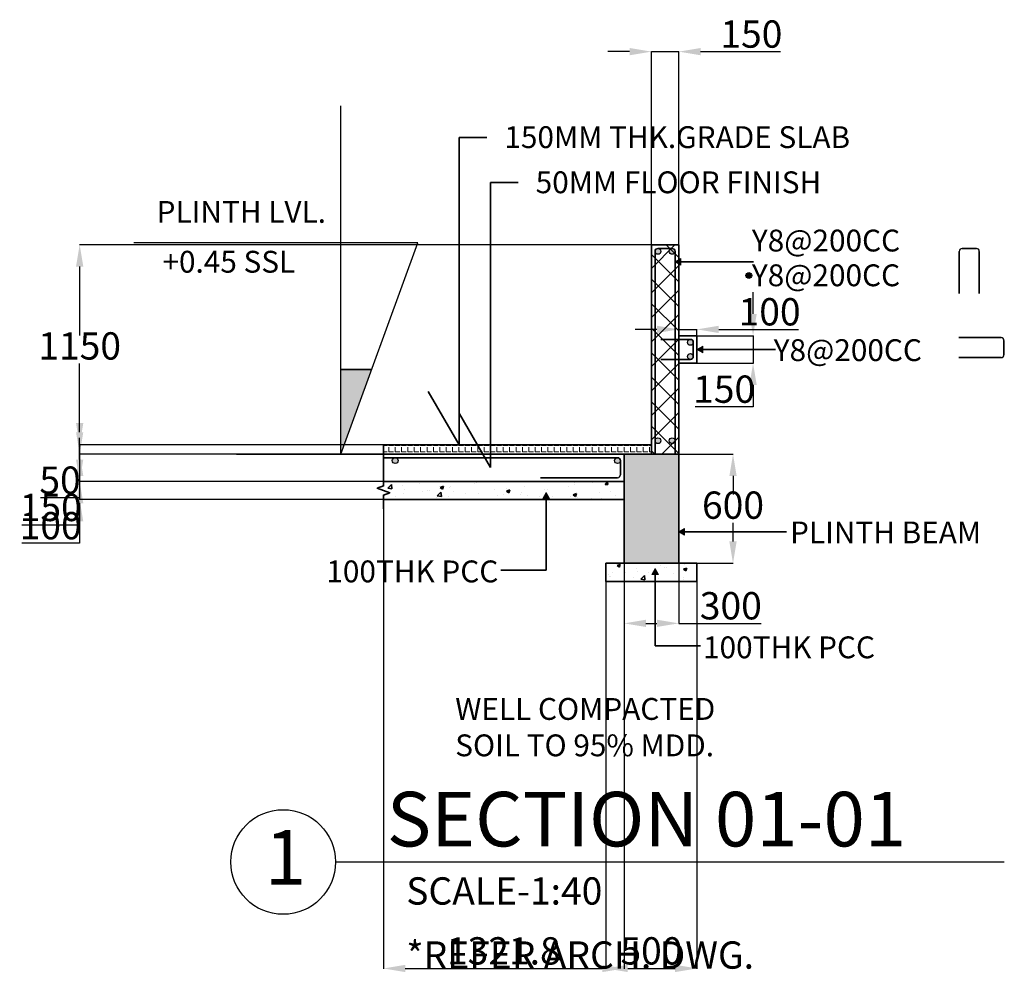
# Model space of a CAD drawing. Units: millimetres. Extents: x -174 to 32373, y 27344 to 53129.
# Tile 1 of 7: x -174 to 5234, y 30305 to 35540. Entities that reach past the tile are written whole.
import ezdxf

# ---------------------------------------------------------------- set-up
doc = ezdxf.new("R2010")
doc.units = ezdxf.units.MM
doc.header["$LTSCALE"] = 50
for name, color, linetype, lineweight in [('S-ANNO-DIMS', 2, 'Continuous', 18), ('S-ANNO-SYMB', 4, 'Continuous', 25), ('S-ANNO-TEXT', 3, 'Continuous', 18), ('S-DETL', 7, 'Continuous', 35), ('S-PATT', 8, 'Continuous', 13), ('S-REIN', 1, 'Continuous', 25)]:
    doc.layers.add(name, color=color, linetype=linetype, lineweight=lineweight)
doc.styles.get("Standard").update_dxf_attribs({"font": 'arial.ttf'})
doc.dimstyles.new('ISO-25', dxfattribs={"dimtxt": 150, "dimasz": 120, "dimexe": 1.25, "dimexo": 0.625, "dimtad": 1, "dimtih": 1, "dimtoh": 1, "dimdec": 0, "dimtxsty": 'Standard', "dimcen": 2.5, "dimadec": 0, "dimazin": 0, "dimtfac": 1, "dimtdec": 0, "dimtmove": 0, "dimatfit": 3, "dimfxl": 1, "dimarcsym": 0})

# ---------------------------------------------------------------- blocks, each defined once
blk = doc.blocks.new('*D30')
at = {"layer": 'Defpoints', "color": 0, "transparency": 16777216}
for p in [(3445.7, 33802.9), (3545.7, 33838.2), (3545.7, 33802.9)]:
    blk.add_point(p, dxfattribs=at)
at = {"layer": 'S-ANNO-DIMS', "color": 0, "lineweight": -2, "transparency": 16777216}
for p, q in [((3325.7, 33838.2), (3205.7, 33838.2)), ((3445.7, 33803.6), (3445.7, 33839.5)), ((3445.7, 33838.2), (3545.7, 33838.2)), ((3545.7, 33803.6), (3545.7, 33839.5)), ((3665.7, 33838.2), (4103.8, 33838.2))]:
    blk.add_line(p, q, dxfattribs=at)
at = {"layer": 'S-ANNO-DIMS', "color": 0, "transparency": 16777216}
for points in [[(3325.7, 33858.2), (3325.7, 33818.2), (3445.7, 33838.2)], [(3665.7, 33858.2), (3665.7, 33818.2), (3545.7, 33838.2)]]:
    blk.add_solid(points, dxfattribs=at)
at = {"layer": 'S-ANNO-DIMS', "color": 0, "transparency": 16777216, "insert": (3944.8, 33915.4), "char_height": 150, "attachment_point": 5}
blk.add_mtext('100', dxfattribs=at)
blk = doc.blocks.new('*D31')
at = {"layer": 'Defpoints', "color": 0, "transparency": 16777216}
for p in [(3545.7, 33802.9), (3545.7, 33652.9), (3854.2, 33652.9)]:
    blk.add_point(p, dxfattribs=at)
at = {"layer": 'S-ANNO-DIMS', "color": 0, "lineweight": -2, "transparency": 16777216}
for p, q in [((3854.2, 33922.9), (3854.2, 34042.9)), ((3546.4, 33802.9), (3855.5, 33802.9)), ((3854.2, 33802.9), (3854.2, 33652.9)), ((3546.4, 33652.9), (3855.5, 33652.9)), ((3854.2, 33532.9), (3854.2, 33412.9)), ((3854.2, 33412.9), (3536.8, 33412.9))]:
    blk.add_line(p, q, dxfattribs=at)
at = {"layer": 'S-ANNO-DIMS', "color": 0, "transparency": 16777216}
for points in [[(3834.2, 33922.9), (3874.2, 33922.9), (3854.2, 33802.9)], [(3834.2, 33532.9), (3874.2, 33532.9), (3854.2, 33652.9)]]:
    blk.add_solid(points, dxfattribs=at)
at = {"layer": 'S-ANNO-DIMS', "color": 0, "transparency": 16777216, "insert": (3695.2, 33490.2), "char_height": 150, "attachment_point": 5}
blk.add_mtext('150', dxfattribs=at)
blk = doc.blocks.new('*D32')
at = {"layer": 'Defpoints', "color": 0, "transparency": 16777216}
for p in [(3445.7, 33152.9), (3743.9, 33152.9), (3445.7, 32552.9)]:
    blk.add_point(p, dxfattribs=at)
at = {"layer": 'S-ANNO-DIMS', "color": 0, "lineweight": -2, "transparency": 16777216}
for p, q in [((3446.4, 33152.9), (3745.1, 33152.9)), ((3743.9, 33032.9), (3743.9, 32930.2)), ((3743.9, 32672.9), (3743.9, 32775.7)), ((3446.4, 32552.9), (3745.1, 32552.9))]:
    blk.add_line(p, q, dxfattribs=at)
at = {"layer": 'S-ANNO-DIMS', "color": 0, "transparency": 16777216}
for points in [[(3723.9, 33032.9), (3763.9, 33032.9), (3743.9, 33152.9)], [(3723.9, 32672.9), (3763.9, 32672.9), (3743.9, 32552.9)]]:
    blk.add_solid(points, dxfattribs=at)
at = {"layer": 'S-ANNO-DIMS', "color": 0, "transparency": 16777216, "insert": (3743.9, 32852.9), "char_height": 150, "attachment_point": 5}
blk.add_mtext('600', dxfattribs=at)
blk = doc.blocks.new('*D33')
at = {"layer": 'Defpoints', "color": 0, "transparency": 16777216}
for p in [(3145.7, 32552.9), (3445.7, 32552.9), (3445.7, 32222.8)]:
    blk.add_point(p, dxfattribs=at)
at = {"layer": 'S-ANNO-DIMS', "color": 0, "lineweight": -2, "transparency": 16777216}
for p, q in [((3145.7, 32552.3), (3145.7, 32221.6)), ((3445.7, 32552.3), (3445.7, 32221.6)), ((3265.7, 32222.8), (3325.7, 32222.8)), ((3445.7, 32222.8), (3897.8, 32222.8))]:
    blk.add_line(p, q, dxfattribs=at)
at = {"layer": 'S-ANNO-DIMS', "color": 0, "transparency": 16777216}
for points in [[(3265.7, 32242.8), (3265.7, 32202.8), (3145.7, 32222.8)], [(3325.7, 32242.8), (3325.7, 32202.8), (3445.7, 32222.8)]]:
    blk.add_solid(points, dxfattribs=at)
at = {"layer": 'S-ANNO-DIMS', "color": 0, "transparency": 16777216, "insert": (3731.8, 32300.1), "char_height": 150, "attachment_point": 5}
blk.add_mtext('300', dxfattribs=at)
blk = doc.blocks.new('LEVEL-MARK')
for p, q in [((1136.3, 0), (1136.3, 1914)), ((1559.1, 1161.7), (0, 1161.7)), ((1136.3, 0), (1559.1, 1161.7))]:
    blk.add_line(p, q)
blk = doc.blocks.new('SECTION-MARK')
blk.add_line((574.9, 287.5), (4248.3, 287.5))
blk.add_circle((287.5, 287.5), 287.5)
blk = doc.blocks.new('*D60')
at = {"layer": 'Defpoints', "color": 0, "transparency": 16777216}
for p in [(155.2, 33152.9), (1824, 33202.9), (3145.7, 33152.9)]:
    blk.add_point(p, dxfattribs=at)
at = {"layer": 'S-ANNO-DIMS', "color": 0, "lineweight": -2, "transparency": 16777216}
for p, q in [((155.2, 33322.9), (155.2, 33442.9)), ((1823.3, 33202.9), (153.9, 33202.9)), ((3145.1, 33152.9), (153.9, 33152.9)), ((155.2, 33202.9), (155.2, 33152.9)), ((155.2, 33032.9), (155.2, 32912.9)), ((155.2, 32912.9), (-59.8, 32912.9))]:
    blk.add_line(p, q, dxfattribs=at)
at = {"layer": 'S-ANNO-DIMS', "color": 0, "transparency": 16777216}
for points in [[(135.2, 33322.9), (175.2, 33322.9), (155.2, 33202.9)], [(135.2, 33032.9), (175.2, 33032.9), (155.2, 33152.9)]]:
    blk.add_solid(points, dxfattribs=at)
at = {"layer": 'S-ANNO-DIMS', "color": 0, "transparency": 16777216, "insert": (47.4, 32990.2), "char_height": 150, "attachment_point": 5}
blk.add_mtext('50', dxfattribs=at)
blk = doc.blocks.new('*D61')
at = {"layer": 'Defpoints', "color": 0, "transparency": 16777216}
for p in [(3145.7, 33152.9), (155.2, 33002.9), (1824, 33002.9)]:
    blk.add_point(p, dxfattribs=at)
at = {"layer": 'S-ANNO-DIMS', "color": 0, "lineweight": -2, "transparency": 16777216}
for p, q in [((155.2, 33272.9), (155.2, 33392.9)), ((3145.1, 33152.9), (153.9, 33152.9)), ((155.2, 33152.9), (155.2, 33002.9)), ((1823.3, 33002.9), (153.9, 33002.9)), ((155.2, 32882.9), (155.2, 32762.9)), ((155.2, 32762.9), (-162.2, 32762.9))]:
    blk.add_line(p, q, dxfattribs=at)
at = {"layer": 'S-ANNO-DIMS', "color": 0, "transparency": 16777216}
for points in [[(135.2, 33272.9), (175.2, 33272.9), (155.2, 33152.9)], [(135.2, 32882.9), (175.2, 32882.9), (155.2, 33002.9)]]:
    blk.add_solid(points, dxfattribs=at)
at = {"layer": 'S-ANNO-DIMS', "color": 0, "transparency": 16777216, "insert": (-3.8, 32840.2), "char_height": 150, "attachment_point": 5}
blk.add_mtext('150', dxfattribs=at)
blk = doc.blocks.new('*D62')
at = {"layer": 'Defpoints', "color": 0, "transparency": 16777216}
for p in [(1824, 33002.9), (155.2, 32902.9), (1824, 32902.9)]:
    blk.add_point(p, dxfattribs=at)
at = {"layer": 'S-ANNO-DIMS', "color": 0, "lineweight": -2, "transparency": 16777216}
for p, q in [((155.2, 33122.9), (155.2, 33242.9)), ((1823.3, 33002.9), (153.9, 33002.9)), ((155.2, 33002.9), (155.2, 32902.9)), ((1823.3, 32902.9), (153.9, 32902.9)), ((155.2, 32782.9), (155.2, 32662.9)), ((155.2, 32662.9), (-162.2, 32662.9))]:
    blk.add_line(p, q, dxfattribs=at)
at = {"layer": 'S-ANNO-DIMS', "color": 0, "transparency": 16777216}
for points in [[(135.2, 33122.9), (175.2, 33122.9), (155.2, 33002.9)], [(135.2, 32782.9), (175.2, 32782.9), (155.2, 32902.9)]]:
    blk.add_solid(points, dxfattribs=at)
at = {"layer": 'S-ANNO-DIMS', "color": 0, "transparency": 16777216, "insert": (-3.8, 32740.2), "char_height": 150, "attachment_point": 5}
blk.add_mtext('100', dxfattribs=at)
blk = doc.blocks.new('*D63')
at = {"layer": 'Defpoints', "color": 0, "transparency": 16777216}
for p in [(1824, 32902.9), (3145.7, 32902.9), (3145.7, 30326.4)]:
    blk.add_point(p, dxfattribs=at)
at = {"layer": 'S-ANNO-DIMS', "color": 0, "lineweight": -2, "transparency": 16777216}
for p, q in [((1824, 32902.3), (1824, 30325.2)), ((3145.7, 32902.3), (3145.7, 30325.2)), ((1944, 30326.4), (3025.7, 30326.4))]:
    blk.add_line(p, q, dxfattribs=at)
at = {"layer": 'S-ANNO-DIMS', "color": 0, "transparency": 16777216}
for points in [[(1944, 30346.4), (1944, 30306.4), (1824, 30326.4)], [(3025.7, 30346.4), (3025.7, 30306.4), (3145.7, 30326.4)]]:
    blk.add_solid(points, dxfattribs=at)
at = {"layer": 'S-ANNO-DIMS', "color": 0, "transparency": 16777216, "insert": (2484.9, 30403.7), "char_height": 150, "attachment_point": 5}
blk.add_mtext('1321.8', dxfattribs=at)
blk = doc.blocks.new('*D64')
at = {"layer": 'Defpoints', "color": 0, "transparency": 16777216}
for p in [(3045.7, 32452.9), (3545.7, 32452.9), (3545.7, 30326.4)]:
    blk.add_point(p, dxfattribs=at)
at = {"layer": 'S-ANNO-DIMS', "color": 0, "lineweight": -2, "transparency": 16777216}
for p, q in [((3045.7, 32452.3), (3045.7, 30325.2)), ((3545.7, 32452.3), (3545.7, 30325.2)), ((3165.7, 30326.4), (3425.7, 30326.4))]:
    blk.add_line(p, q, dxfattribs=at)
at = {"layer": 'S-ANNO-DIMS', "color": 0, "transparency": 16777216}
for points in [[(3165.7, 30346.4), (3165.7, 30306.4), (3045.7, 30326.4)], [(3425.7, 30346.4), (3425.7, 30306.4), (3545.7, 30326.4)]]:
    blk.add_solid(points, dxfattribs=at)
at = {"layer": 'S-ANNO-DIMS', "color": 0, "transparency": 16777216, "insert": (3295.7, 30403.6), "char_height": 150, "attachment_point": 5}
blk.add_mtext('500', dxfattribs=at)
blk = doc.blocks.new('*D65')
at = {"layer": 'Defpoints', "color": 0, "transparency": 16777216}
for p in [(3295.7, 34302.9), (155.2, 33152.9), (3145.7, 33152.9)]:
    blk.add_point(p, dxfattribs=at)
at = {"layer": 'S-ANNO-DIMS', "color": 0, "lineweight": -2, "transparency": 16777216}
for p, q in [((3295.1, 34302.9), (153.9, 34302.9)), ((155.2, 34182.9), (155.2, 33805.2)), ((155.2, 33272.9), (155.2, 33650.7)), ((3145.1, 33152.9), (153.9, 33152.9))]:
    blk.add_line(p, q, dxfattribs=at)
at = {"layer": 'S-ANNO-DIMS', "color": 0, "transparency": 16777216}
for points in [[(135.2, 34182.9), (175.2, 34182.9), (155.2, 34302.9)], [(135.2, 33272.9), (175.2, 33272.9), (155.2, 33152.9)]]:
    blk.add_solid(points, dxfattribs=at)
at = {"layer": 'S-ANNO-DIMS', "color": 0, "transparency": 16777216, "insert": (155.2, 33727.9), "char_height": 150, "attachment_point": 5}
blk.add_mtext('1150', dxfattribs=at)
blk = doc.blocks.new('*D66')
at = {"layer": 'Defpoints', "color": 0, "transparency": 16777216}
for p in [(3445.7, 35364.4), (3295.7, 34302.9), (3445.7, 34302.9)]:
    blk.add_point(p, dxfattribs=at)
at = {"layer": 'S-ANNO-DIMS', "color": 0, "lineweight": -2, "transparency": 16777216}
for p, q in [((3175.7, 35364.4), (3055.7, 35364.4)), ((3295.7, 34303.6), (3295.7, 35365.7)), ((3295.7, 35364.4), (3445.7, 35364.4)), ((3445.7, 34303.6), (3445.7, 35365.7)), ((3565.7, 35364.4), (4003.8, 35364.4))]:
    blk.add_line(p, q, dxfattribs=at)
at = {"layer": 'S-ANNO-DIMS', "color": 0, "transparency": 16777216}
for points in [[(3175.7, 35384.4), (3175.7, 35344.4), (3295.7, 35364.4)], [(3565.7, 35384.4), (3565.7, 35344.4), (3445.7, 35364.4)]]:
    blk.add_solid(points, dxfattribs=at)
at = {"layer": 'S-ANNO-DIMS', "color": 0, "transparency": 16777216, "insert": (3844.8, 35441.6), "char_height": 150, "attachment_point": 5}
blk.add_mtext('150', dxfattribs=at)

msp = doc.modelspace()

# ---------------------------------------------------------------- hatches: boundary and pattern name
at = {"layer": 'S-ANNO-SYMB'}
h = msp.add_hatch(color=256, dxfattribs=at)
h.dxf.hatch_style = 1
h.paths.add_polyline_path([(1588.98, 33152.95), (1758.2, 33617.86), (1588.98, 33617.86)])
at = {"layer": 'S-ANNO-TEXT'}
h = msp.add_hatch(color=256, dxfattribs=at)
h.dxf.hatch_style = 1
h.paths.add_polyline_path([(3425.75, 34209.89), (3457.5, 34191.56), (3457.5, 34228.23)])
h = msp.add_hatch(color=256, dxfattribs=at)
h.dxf.hatch_style = 1
h.paths.add_polyline_path([(3846.81, 34134.35, 1), (3814.81, 34134.35, 1)])
h = msp.add_hatch(color=256, dxfattribs=at)
h.dxf.hatch_style = 1
h.paths.add_polyline_path([(3545.75, 33727.95), (3577.5, 33709.61), (3577.5, 33746.28)])
h = msp.add_hatch(color=256, dxfattribs=at)
h.dxf.hatch_style = 1
h.paths.add_polyline_path([(2717.97, 32941.04), (2699.64, 32909.28), (2736.3, 32909.28)])
h = msp.add_hatch(color=256, dxfattribs=at)
h.dxf.hatch_style = 1
h.paths.add_polyline_path([(3445.75, 32726.27), (3477.5, 32707.93), (3477.5, 32744.6)])
h = msp.add_hatch(color=256, dxfattribs=at)
h.dxf.hatch_style = 1
h.paths.add_polyline_path([(3315.93, 32523.71), (3297.6, 32491.96), (3334.26, 32491.96)])
at = {"layer": 'S-PATT'}
h = msp.add_hatch(dxfattribs=at)
h.set_pattern_fill('ANSI37', color=256, scale=30)
h.set_pattern_definition([(45, (-34922.54, -14821.09), (-67.35192, 67.35192), []), (135, (-34922.54, -14821.09), (-67.35192, -67.35192), [])])
h.paths.add_polyline_path([(3445.75, 34302.95), (3295.75, 34302.95), (3295.75, 33152.95), (3445.75, 33152.95)])
h = msp.add_hatch(color=256, dxfattribs=at)
h.dxf.hatch_style = 1
h.paths.add_polyline_path([(3347.75, 34266.95, 1), (3315.75, 34266.95, 1)])
h.paths.add_polyline_path([(3425.75, 34266.95, 0.4142136), (3409.75, 34282.95, 0.4142136), (3393.75, 34266.95, 1)])
h.paths.add_polyline_path([(3525.75, 33766.95, 1), (3493.75, 33766.95, 1)])
h.paths.add_polyline_path([(3525.75, 33688.95, 1), (3493.75, 33688.95, 1)])
h.paths.add_polyline_path([(3425.75, 33226.45, 1), (3393.75, 33226.45, 1)])
h.paths.add_polyline_path([(3347.75, 33226.45, 1), (3315.75, 33226.45, 1)])
h.paths.add_polyline_path([(3125.75, 33116.95, 1), (3093.75, 33116.95, 1)])
h.paths.add_polyline_path([(1904.55, 33116.95, 1), (1872.55, 33116.95, 1)])
h = msp.add_hatch(dxfattribs=at)
h.set_pattern_fill('ANGLE', color=256, scale=5)
h.set_pattern_definition([(0, (-34922.54, -14821.088), (0, 34.925), [25.4, -9.525]), (90, (-34922.54, -14821.088), (-34.925, 2e-15), [25.4, -9.525])])
h.paths.add_polyline_path([(3145.75, 33152.95), (3295.75, 33152.95), (3295.75, 33202.95), (1823.96, 33202.95), (1823.96, 33152.95)])
h = msp.add_hatch(color=256, dxfattribs=at)
h.dxf.hatch_style = 1
h.paths.add_polyline_path([(3145.75, 32552.95), (3445.75, 32552.95), (3445.75, 33152.95), (3145.75, 33152.95)])

# ---------------------------------------------------------------- linework, layer by layer
at = {"layer": 'S-ANNO-TEXT'}
for p, q in [((2717.97, 32941.04), (2717.97, 32941.04)), ((3315.93, 32523.71), (3315.93, 32523.71))]:
    msp.add_line(p, q, dxfattribs=at)
for points in [[(3425.75, 34209.89), (3457.5, 34191.56), (3457.5, 34228.23)], [(3545.75, 33727.95), (3577.5, 33709.61), (3577.5, 33746.28)], [(2717.97, 32941.04), (2699.64, 32909.28), (2736.3, 32909.28)], [(3445.75, 32726.27), (3477.5, 32707.93), (3477.5, 32744.6)], [(3315.93, 32523.71), (3297.6, 32491.96), (3334.26, 32491.96)]]:
    msp.add_lwpolyline(points, close=True, dxfattribs=at)
at = {"layer": 'S-DETL'}
for p, q in [((2239.41, 33202.95), (2239.41, 34893.4)), ((2239.41, 34893.4), (2391.57, 34893.4)), ((2411.35, 33079.08), (2411.35, 34645.29)), ((2411.35, 34645.29), (2563.51, 34645.29)), ((3295.75, 33152.95), (3295.75, 34302.95)), ((3445.75, 34302.95), (3295.75, 34302.95)), ((3445.75, 33152.95), (3445.75, 34302.95)), ((3315.75, 33152.95), (3315.75, 34266.95)), ((3409.75, 34282.95), (3331.75, 34282.95)), ((3425.75, 33152.95), (3425.75, 34266.95)), ((4986.55, 34035.6), (4986.55, 34266.95)), ((5080.55, 34282.95), (5002.55, 34282.95)), ((5096.55, 34035.6), (5096.55, 34266.95)), ((3457.5, 34209.89), (3856.75, 34209.89)), ((3445.75, 33802.95), (3545.75, 33802.95)), ((3545.75, 33652.95), (3545.75, 33802.95)), ((3348.16, 33782.95), (3509.75, 33782.95)), ((3525.75, 33688.95), (3525.75, 33766.95)), ((4984.7, 33792.86), (5216.05, 33792.86)), ((5232.05, 33698.86), (5232.05, 33776.86)), ((3577.5, 33727.95), (3976.75, 33727.95)), ((3348.16, 33672.95), (3509.75, 33672.95)), ((3445.75, 33652.95), (3545.75, 33652.95)), ((4984.7, 33682.86), (5216.05, 33682.86)), ((1588.98, 33617.86), (1758.2, 33617.86)), ((2239.41, 33202.95), (2069.4, 33497.41)), ((2411.35, 33079.08), (2241.34, 33373.55)), ((3145.75, 33152.95), (1016.41, 33152.95)), ((3295.75, 33202.95), (1823.96, 33202.95)), ((3145.75, 33152.95), (3445.75, 33152.95)), ((3145.75, 32552.95), (3145.75, 33152.95)), ((3295.75, 33152.95), (3295.75, 33202.95)), ((3445.75, 33152.95), (3445.75, 32552.95)), ((3109.75, 33132.95), (1823.96, 33132.95)), ((3125.75, 33038.95), (3125.75, 33116.95)), ((3145.75, 33002.95), (1823.96, 33002.95)), ((1976.17, 33001.36), (1976.17, 33001.36)), ((2022.26, 32993.08), (2022.26, 32993.08)), ((2333.29, 32996.45), (2333.29, 32996.45)), ((3109.75, 33022.95), (2686.05, 33022.95)), ((2756.25, 32998.33), (2756.25, 32998.33)), ((2859.26, 33002.21), (2859.88, 33002.95)), ((2859.26, 33002.21), (2874.44, 33000.88)), ((2874.45, 33000.88), (2874.07, 33002.95)), ((2972.37, 32994.89), (2972.37, 32994.89)), ((3041.45, 32986.27), (3053.69, 33000.87)), ((3056.63, 32984.94), (3053.7, 33000.86)), ((3090.67, 33002.95), (3091.65, 33002.29)), ((3091.65, 33002.28), (3091.88, 33002.95)), ((1802.92, 32961.84), (1802.92, 32961.84)), ((1828.04, 32975.94), (1828.04, 32975.94)), ((1848.14, 32965.05), (1867.93, 32985.67)), ((1848.15, 32965.04), (1870.74, 32961.54)), ((1862.48, 32972.04), (1862.48, 32972.04)), ((1870.74, 32961.55), (1867.93, 32985.67)), ((1926.07, 32980.41), (1926.07, 32980.41)), ((1938.51, 32956.11), (1938.51, 32956.11)), ((2037.03, 32945.59), (2037.03, 32945.59)), ((2063.77, 32955.19), (2063.77, 32955.19)), ((2074.1, 32950.38), (2074.1, 32950.38)), ((2119.22, 32923.01), (2139.01, 32943.63)), ((2135.54, 32969.57), (2148.17, 32961.05)), ((2135.56, 32969.62), (2153.34, 32976.44)), ((2141.82, 32919.51), (2139.01, 32943.63)), ((2148.18, 32961.05), (2153.33, 32976.4)), ((2185.16, 32971.02), (2185.16, 32971.02)), ((2194.19, 32973.07), (2194.19, 32973.07)), ((2209.69, 32944.65), (2209.69, 32944.65)), ((2322.48, 32989.33), (2322.48, 32989.33)), ((2345.28, 32938.92), (2345.28, 32938.92)), ((2436.06, 32956.17), (2436.06, 32956.17)), ((2499.64, 32964.54), (2499.64, 32964.54)), ((2500.57, 32949.23), (2513.2, 32940.7)), ((2500.59, 32949.27), (2518.37, 32956.1)), ((2513.21, 32940.7), (2518.36, 32956.05)), ((2581.73, 32941.7), (2581.73, 32941.7)), ((2595.84, 32977.21), (2595.84, 32977.21)), ((2710.03, 32957.96), (2710.03, 32957.96)), ((2726.56, 32958.41), (2726.56, 32958.41)), ((2841.95, 32977.01), (2841.95, 32977.01)), ((2874.69, 32983.84), (2874.69, 32983.84)), ((3009.63, 32940.3), (3009.63, 32940.3)), ((3041.45, 32986.27), (3056.63, 32984.94)), ((3073.22, 32948.67), (3073.22, 32948.67)), ((3145.75, 32902.95), (1823.96, 32902.95)), ((1888.91, 32920.17), (1888.91, 32920.17)), ((1931.85, 32936.14), (1931.85, 32936.14)), ((1993.73, 32902.95), (1995.83, 32905.44)), ((1996.3, 32902.95), (1995.84, 32905.44)), ((2115.86, 32914.02), (2115.86, 32914.02)), ((2119.23, 32923), (2141.82, 32919.5)), ((2179.44, 32922.39), (2179.44, 32922.39)), ((2275.64, 32935.05), (2275.64, 32935.05)), ((2319.39, 32904.78), (2319.39, 32904.78)), ((2430.3, 32907.56), (2430.3, 32907.56)), ((2451.32, 32923.82), (2451.32, 32923.82)), ((2480.87, 32933.19), (2480.87, 32933.19)), ((2578.43, 32932.98), (2578.43, 32932.98)), ((2616.46, 32927.47), (2616.46, 32927.47)), ((2682.59, 32921.72), (2682.59, 32921.72)), ((2717.97, 32909.28), (2717.97, 32515.74)), ((2736.14, 32887.6), (2736.14, 32887.6)), ((2752.05, 32921.74), (2752.05, 32921.74)), ((2753.02, 32906.52), (2753.02, 32906.52)), ((2849.22, 32919.18), (2849.22, 32919.18)), ((2865.6, 32928.88), (2878.23, 32920.36)), ((2865.62, 32928.93), (2883.41, 32935.76)), ((2878.24, 32920.36), (2883.39, 32935.71)), ((2887.64, 32916.01), (2887.64, 32916.01)), ((2969.28, 32910.34), (2969.28, 32910.34)), ((3023.23, 32910.28), (3023.23, 32910.28)), ((3097.57, 32926.6), (3097.57, 32926.6)), ((3477.5, 32726.27), (4037.33, 32726.27)), ((2717.97, 32515.74), (2467.96, 32515.74)), ((3045.75, 32452.95), (3045.75, 32552.95)), ((3045.75, 32552.95), (3145.75, 32552.95)), ((3082.13, 32503.82), (3082.13, 32503.82)), ((3107.03, 32540.17), (3119.66, 32531.64)), ((3107.05, 32540.21), (3124.83, 32547.04)), ((3119.66, 32531.64), (3124.81, 32546.99)), ((3144.96, 32510.12), (3144.96, 32510.12)), ((3445.75, 32552.95), (3145.75, 32552.95)), ((3214.06, 32522.87), (3214.06, 32522.87)), ((3220.57, 32505.73), (3220.57, 32505.73)), ((3280.55, 32504.4), (3280.55, 32504.4)), ((3344.47, 32540.75), (3344.47, 32540.75)), ((3368.7, 32531.16), (3368.7, 32531.16)), ((3379.52, 32532.08), (3379.52, 32532.08)), ((3445.75, 32552.95), (3545.75, 32552.95)), ((3472.06, 32519.82), (3484.69, 32511.3)), ((3472.08, 32519.87), (3489.86, 32526.7)), ((3475.71, 32544.74), (3475.71, 32544.74)), ((3484.69, 32511.3), (3489.84, 32526.65)), ((3545.75, 32552.95), (3545.75, 32452.95)), ((3545.75, 32452.95), (3045.75, 32452.95)), ((3059.32, 32489.93), (3059.32, 32489.93)), ((3062.92, 32481.73), (3062.92, 32481.73)), ((3072.44, 32480.3), (3072.44, 32480.3)), ((3155.52, 32502.59), (3155.52, 32502.59)), ((3198.51, 32476.01), (3198.51, 32476.01)), ((3237.21, 32465.37), (3257, 32485.99)), ((3237.22, 32465.36), (3259.81, 32461.86)), ((3259.81, 32461.87), (3257, 32485.99)), ((3315.93, 32491.96), (3315.93, 32098.41)), ((3334.1, 32470.28), (3334.1, 32470.28)), ((3341.38, 32456.2), (3341.38, 32456.2)), ((3416.14, 32498.67), (3416.14, 32498.67)), ((3469.68, 32472.46), (3469.68, 32472.46)), ((3469.69, 32464.55), (3469.69, 32464.55)), ((3315.93, 32098.41), (3565.94, 32098.41))]:
    msp.add_line(p, q, dxfattribs=at)
msp.add_lwpolyline([(1823.96, 33202.95), (1823.96, 32977.95), (1789.61, 32965.45), (1858.3, 32940.45), (1823.96, 32927.95), (1823.96, 32852.95)], dxfattribs=at)
at = {"layer": 'S-REIN'}
for centre in [(3331.75, 34266.95), (3409.75, 34266.95), (3830.81, 34134.35), (3509.75, 33766.95), (3509.75, 33688.95), (3331.75, 33226.45), (3409.75, 33226.45), (1888.55, 33116.95), (3109.75, 33116.95)]:
    msp.add_circle(centre, 16, dxfattribs=at)
for centre, start, end in [((3331.75, 34266.95), 90, 180), ((3409.75, 34266.95), 0, 90), ((5002.55, 34266.95), 90, 180), ((5080.55, 34266.95), 0, 90), ((3509.75, 33766.95), 0, 90), ((5216.05, 33776.86), 0, 90), ((5216.05, 33698.86), 270, 0), ((3509.75, 33688.95), 270, 0), ((3109.75, 33116.95), 0, 90), ((3109.75, 33038.95), 270, 0)]:
    msp.add_arc(centre, 16, start, end, dxfattribs=at)

# ---------------------------------------------------------------- block references
at = {"layer": 'S-ANNO-SYMB'}
for name, p in [('LEVEL-MARK', (452.67, 33152.95)), ('SECTION-MARK', (985.68, 30623.9))]:
    msp.add_blockref(name, p, dxfattribs=at)

# ---------------------------------------------------------------- texts
at = {"layer": 'S-ANNO-TEXT'}
for s, width, insert, char_height, attachment_point in [('150MM THK.GRADE SLAB', 2900.7274, (2487.95, 34954.52), 120, 1), ('50MM FLOOR FINISH', 2900.7274, (2659.89, 34706.41), 120, 1), ('PLINTH LVL.', 1913.0414, (578.07, 34543.88), 120, 1), ('Y8@200CC', 1913.0414, (3847.51, 34386.29), 120, 1), ('+0.45 SSL', 1913.0414, (609.74, 34269.9), 120, 1), ('Y8@200CC', 1913.0414, (3847.51, 34195.35), 120, 1), ('Y8@200CC', 1913.0414, (3967.51, 33784.03), 120, 1), ('PLINTH BEAM', 1913.0414, (4057.37, 32782.35), 120, 1), ('100THK PCC', 1913.0414, (2454.77, 32568.25), 120, 3), ('100THK PCC', 1913.0414, (3579.13, 32150.92), 120, 1), ('WELL COMPACTED\\PSOIL TO 95% MDD.', 1913.0414, (2218.1, 31812.41), 120, 1), ('SECTION 01-01', 6501.8432, (1842.16, 31296.91), 300, 1), ('1', 6501.8432, (1172.6, 31086.73), 300, 1), ('SCALE-1:40', 1913.0414, (1948.96, 30827.3), 150, 1), ('*REFER ARCH. DWG.', 2642.4337, (1948.96, 30475.12), 150, 1)]:
    msp.add_mtext_dynamic_manual_height_columns(s, width=width, gutter_width=12.5, heights=[0], dxfattribs=dict(at, insert=insert, char_height=char_height, attachment_point=attachment_point))

# ---------------------------------------------------------------- dimensions: what is measured, and where the dimension line sits
at = {"layer": 'S-ANNO-DIMS'}
for base, p1, p2, override, picture, middle in [((3445.75, 35364.41), (3295.75, 34302.95), (3445.75, 34302.95), {"dimdec": 0, "dimlfac": 1, "dimrnd": 0, "dimzin": 0, "dimdsep": 46, "dimlunit": 2}, '*D66', (3844.76, 35441.62)), ((3545.75, 33838.22), (3445.75, 33802.95), (3545.75, 33802.95), {"dimclrd": 0, "dimclre": 0, "dimclrt": 0}, '*D30', (3944.76, 33915.43)), ((3145.75, 30326.4), (1823.96, 32902.95), (3145.75, 32902.95), {"dimdec": 1, "dimlfac": 1, "dimrnd": 0, "dimzin": 0, "dimdsep": 46, "dimlunit": 2}, '*D63', (2484.85, 30403.67)), ((3445.75, 32222.81), (3145.75, 32552.95), (3445.75, 32552.95), {"dimclrd": 0, "dimclre": 0, "dimclrt": 0}, '*D33', (3731.77, 32300.07)), ((3545.75, 30326.4), (3045.75, 32452.95), (3545.75, 32452.95), {"dimdec": 0, "dimlfac": 1, "dimrnd": 0, "dimzin": 0, "dimdsep": 46, "dimlunit": 2}, '*D64', (3295.75, 30403.61))]:
    dim = msp.add_linear_dim(base=base, p1=p1, p2=p2, dimstyle='ISO-25', override=override, dxfattribs=at)
    dim.commit()
    dim.dimension.update_dxf_attribs({"geometry": picture, "text_midpoint": middle})
for base, p1, p2, override, picture, middle in [((155.17, 33152.95), (3295.75, 34302.95), (3145.75, 33152.95), {"dimdec": 0, "dimlfac": 1, "dimrnd": 0, "dimzin": 0, "dimdsep": 46, "dimlunit": 2}, '*D65', (155.17, 33727.95)), ((3854.25, 33652.95), (3545.75, 33802.95), (3545.75, 33652.95), {"dimclrd": 0, "dimclre": 0, "dimclrt": 0}, '*D31', (3695.23, 33490.16)), ((155.17, 33152.95), (1823.96, 33202.95), (3145.75, 33152.95), {"dimdec": 0, "dimlfac": 1, "dimrnd": 0, "dimzin": 0, "dimdsep": 46, "dimlunit": 2}, '*D60', (47.36, 32990.16)), ((155.17, 33002.95), (3145.75, 33152.95), (1823.96, 33002.95), {"dimdec": 0, "dimlfac": 1, "dimrnd": 0, "dimzin": 0, "dimdsep": 46, "dimlunit": 2}, '*D61', (-3.85, 32840.16)), ((155.17, 32902.95), (1823.96, 33002.95), (1823.96, 32902.95), {"dimdec": 0, "dimlfac": 1, "dimrnd": 0, "dimzin": 0, "dimdsep": 46, "dimlunit": 2}, '*D62', (-3.85, 32740.16)), ((3743.86, 33152.95), (3445.75, 32552.95), (3445.75, 33152.95), {"dimclrd": 0, "dimclre": 0, "dimclrt": 0}, '*D32', (3743.86, 32852.95))]:
    dim = msp.add_linear_dim(base=base, p1=p1, p2=p2, angle=90, dimstyle='ISO-25', override=override, dxfattribs=at)
    dim.commit()
    dim.dimension.update_dxf_attribs({"geometry": picture, "text_midpoint": middle})

doc.saveas('drawing.dxf')
